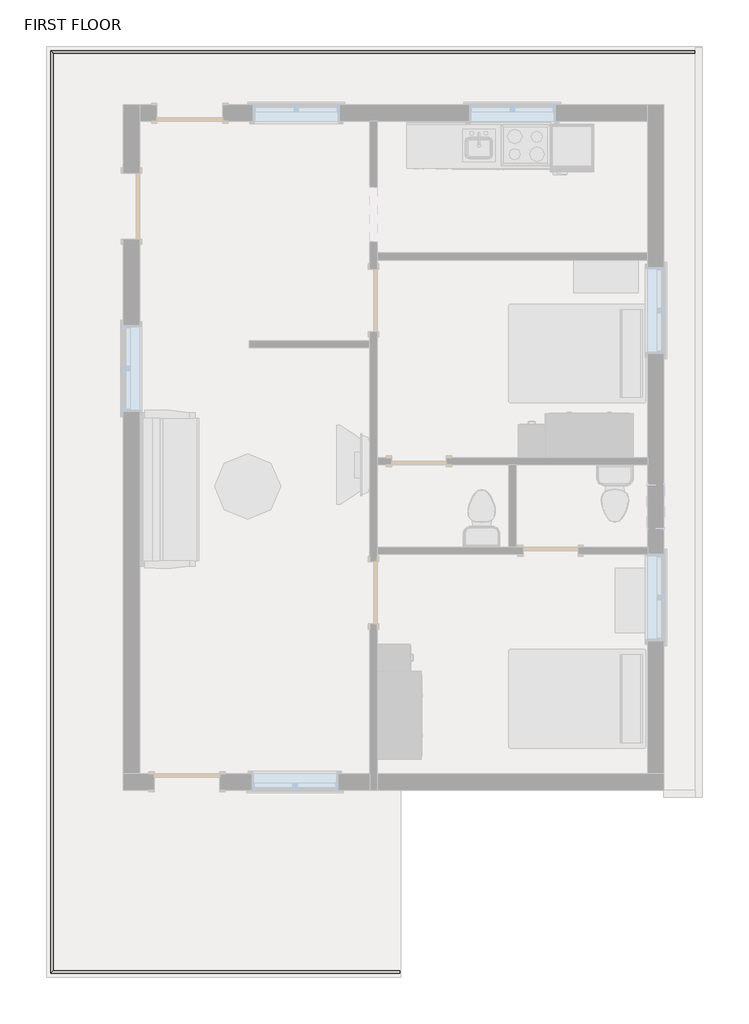
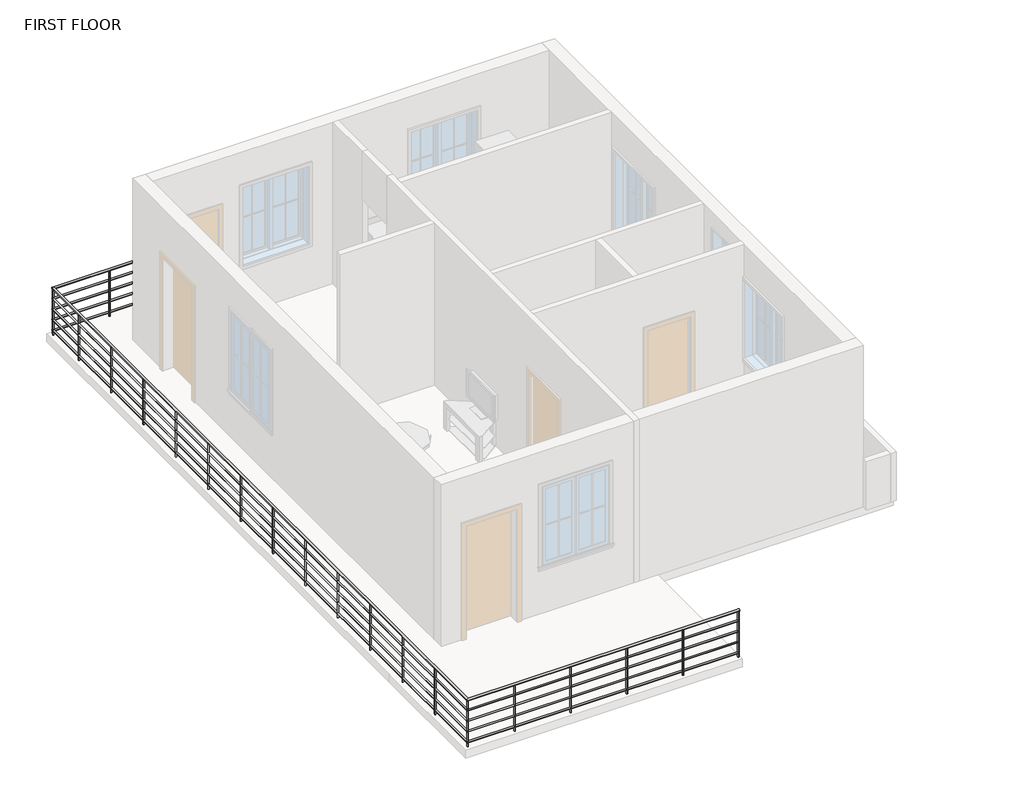
# One storey, part 2 of 3: 1 railing.
"""IFC4 building model written with IfcOpenShell, lengths in millimetres."""

from ifc_helpers import new_model, si_unit, point, frame, frame_2d, origin, place, context, project, spatial, circle_curve, ellipse_curve, trimmed, segment, composite_curve, outline, extrude, element, save
from ifc_brep_helpers import plane_surface, cylinder_surface, advanced_brep

model = new_model("IFC4")

# Units and contexts
model_context = context("Model", 3, world=origin())
ifc_project = project(units=[si_unit("LENGTHUNIT", "METRE", prefix="MILLI")], contexts=[model_context])

# Site, building, storey
site = spatial("IfcSite", under=ifc_project)
building = spatial("IfcBuilding", under=site)
storey = spatial("IfcBuildingStorey", under=building, Name="FIRST FLOOR", Elevation=3200.4)

# Railing
placement = place(None, origin())
element("IfcRailing", 1, ObjectType="900mm Pipe", at=placement, inside=storey, context=model_context, shape_type="SolidModel", body=[
    advanced_brep(
    [(200.9145071, -6925.6741001, 4080.4), (200.9145071, -6965.6741001, 4080.4), (-4655.4544048, -6965.6741001, 4080.4), (-4615.4544048, -6925.6741001, 4080.4), (-4655.4544048, 5865.7351347, 4080.4), (-4615.4544048, 5825.7351347, 4080.4), (4406.9455952, 5825.7351347, 4080.4), (4406.9455952, 5865.7351347, 4080.4)],
    [
        (0, 1, circle_curve(frame((200.9145071, -6945.6741001, 4080.4), z_axis=(1.0, 0.0, 0.0), x_axis=(0.0, -1.0, 0.0)), 20.0)),
        (1, 0, circle_curve(frame((200.9145071, -6945.6741001, 4080.4), z_axis=(1.0, 0.0, 0.0), x_axis=(0.0, -1.0, 0.0)), 20.0)),
        (1, 2),
        (2, 3, ellipse_curve(frame((-4635.4544048, -6945.6741001, 4080.4), z_axis=(0.7071067811865458, -0.7071067811865492, 0.0), x_axis=(0.7071067811865492, 0.7071067811865458, 0.0)), 28.2842712, 20.0)),
        (3, 0),
        (3, 2, ellipse_curve(frame((-4635.4544048, -6945.6741001, 4080.4), z_axis=(0.7071067811865458, -0.7071067811865492, 0.0), x_axis=(0.7071067811865492, 0.7071067811865458, 0.0)), 28.2842712, 20.0)),
        (2, 4),
        (4, 5, ellipse_curve(frame((-4635.4544048, 5845.7351347, 4080.4), z_axis=(-0.7071067811865491, -0.7071067811865459, 0.0), x_axis=(0.7071067811865458, -0.7071067811865491, 0.0)), 28.2842712, 20.0)),
        (5, 3),
        (5, 4, ellipse_curve(frame((-4635.4544048, 5845.7351347, 4080.4), z_axis=(-0.7071067811865491, -0.7071067811865459, 0.0), x_axis=(0.7071067811865458, -0.7071067811865491, 0.0)), 28.2842712, 20.0)),
        (6, 7, circle_curve(frame((4406.9455952, 5845.7351347, 4080.4), z_axis=(1.0, 0.0, 0.0), x_axis=(0.0, 1.0, 0.0)), 20.0)),
        (7, 6, circle_curve(frame((4406.9455952, 5845.7351347, 4080.4), z_axis=(1.0, 0.0, 0.0), x_axis=(0.0, 1.0, 0.0)), 20.0)),
        (4, 7),
        (6, 5),
    ],
    [
        plane_surface(frame((200.9145071, -6945.6741001, 4100.4), z_axis=(1.0, 0.0, 0.0), x_axis=(0.0, -1.0, 0.0))),
        cylinder_surface(frame((200.9145071, -6945.6741001, 4080.4), z_axis=(1.0, 0.0, 0.0), x_axis=(0.0, -1.0, 0.0)), 20.0),
        cylinder_surface(frame((-4635.4544048, -6945.6741001, 4080.4), z_axis=(0.0, -1.0, 0.0), x_axis=(-1.0, 0.0, 0.0)), 20.0),
        plane_surface(frame((4406.9455952, 5845.7351347, 4100.4), z_axis=(1.0, 0.0, 0.0), x_axis=(0.0, 1.0, 0.0))),
        cylinder_surface(frame((-4635.4544048, 5845.7351347, 4080.4), z_axis=(-1.0, 0.0, 0.0), x_axis=(0.0, 1.0, 0.0)), 20.0),
    ],
    [
        (0, [[1, 2]]),
        (1, [[-2, 3, 4, 5]]),
        (1, [[-1, -5, 6, -3]]),
        (2, [[-4, 7, 8, 9]]),
        (2, [[-6, -9, 10, -7]]),
        (3, [[11, 12]]),
        (4, [[-8, 13, -11, 14]]),
        (4, [[-10, -14, -12, -13]]),
    ],
),
    advanced_brep(
    [(200.9145071, -6960.6741001, 3885.4), (200.9145071, -6930.6741001, 3885.4), (4406.9455952, 5860.7351347, 3885.4), (4406.9455952, 5830.7351347, 3885.4), (-4650.4544048, -6960.6741001, 3885.4), (-4620.4544048, -6930.6741001, 3885.4), (-4650.4544048, 5860.7351347, 3885.4), (-4620.4544048, 5830.7351347, 3885.4)],
    [
        (0, 1, circle_curve(frame((200.9145071, -6945.6741001, 3885.4), z_axis=(1.0, 0.0, 0.0), x_axis=(0.0, 1.0, 0.0)), 15.0)),
        (1, 0, circle_curve(frame((200.9145071, -6945.6741001, 3885.4), z_axis=(1.0, 0.0, 0.0), x_axis=(0.0, 1.0, 0.0)), 15.0)),
        (2, 3, circle_curve(frame((4406.9455952, 5845.7351347, 3885.4), z_axis=(1.0, 0.0, 0.0), x_axis=(0.0, -1.0, 0.0)), 15.0)),
        (3, 2, circle_curve(frame((4406.9455952, 5845.7351347, 3885.4), z_axis=(1.0, 0.0, 0.0), x_axis=(0.0, -1.0, 0.0)), 15.0)),
        (0, 4),
        (4, 5, ellipse_curve(frame((-4635.4544048, -6945.6741001, 3885.4), z_axis=(0.7071067811865458, -0.7071067811865492, 0.0), x_axis=(0.7071067811865492, 0.7071067811865458, 0.0)), 21.2132034, 15.0)),
        (5, 1),
        (5, 4, ellipse_curve(frame((-4635.4544048, -6945.6741001, 3885.4), z_axis=(0.7071067811865458, -0.7071067811865492, 0.0), x_axis=(0.7071067811865492, 0.7071067811865458, 0.0)), 21.2132034, 15.0)),
        (4, 6),
        (6, 7, ellipse_curve(frame((-4635.4544048, 5845.7351347, 3885.4), z_axis=(-0.7071067811865491, -0.7071067811865459, 0.0), x_axis=(0.7071067811865458, -0.7071067811865491, 0.0)), 21.2132034, 15.0)),
        (7, 5),
        (7, 6, ellipse_curve(frame((-4635.4544048, 5845.7351347, 3885.4), z_axis=(-0.7071067811865491, -0.7071067811865459, 0.0), x_axis=(0.7071067811865458, -0.7071067811865491, 0.0)), 21.2132034, 15.0)),
        (6, 2),
        (3, 7),
    ],
    [
        plane_surface(frame((200.9145071, -6945.6741001, 3900.4), z_axis=(1.0, 0.0, 0.0), x_axis=(0.0, -1.0, 0.0))),
        plane_surface(frame((4406.9455952, 5845.7351347, 3900.4), z_axis=(1.0, 0.0, 0.0), x_axis=(0.0, 1.0, 0.0))),
        cylinder_surface(frame((200.9145071, -6945.6741001, 3885.4), z_axis=(1.0, 0.0, 0.0), x_axis=(0.0, 1.0, 0.0)), 15.0),
        cylinder_surface(frame((-4635.4544048, -6945.6741001, 3885.4), z_axis=(0.0, -1.0, 0.0), x_axis=(1.0, 0.0, 0.0)), 15.0),
        cylinder_surface(frame((-4635.4544048, 5845.7351347, 3885.4), z_axis=(-1.0, 0.0, 0.0), x_axis=(0.0, -1.0, 0.0)), 15.0),
    ],
    [
        (0, [[1, 2]]),
        (1, [[3, 4]]),
        (2, [[-1, 5, 6, 7]]),
        (2, [[-2, -7, 8, -5]]),
        (3, [[-6, 9, 10, 11]]),
        (3, [[-8, -11, 12, -9]]),
        (4, [[-10, 13, -4, 14]]),
        (4, [[-12, -14, -3, -13]]),
    ],
),
    advanced_brep(
    [(200.9145071, -6960.6741001, 3685.4), (200.9145071, -6930.6741001, 3685.4), (4406.9455952, 5860.7351347, 3685.4), (4406.9455952, 5830.7351347, 3685.4), (-4650.4544048, -6960.6741001, 3685.4), (-4620.4544048, -6930.6741001, 3685.4), (-4650.4544048, 5860.7351347, 3685.4), (-4620.4544048, 5830.7351347, 3685.4)],
    [
        (0, 1, circle_curve(frame((200.9145071, -6945.6741001, 3685.4), z_axis=(1.0, 0.0, 0.0), x_axis=(0.0, 1.0, 0.0)), 15.0)),
        (1, 0, circle_curve(frame((200.9145071, -6945.6741001, 3685.4), z_axis=(1.0, 0.0, 0.0), x_axis=(0.0, 1.0, 0.0)), 15.0)),
        (2, 3, circle_curve(frame((4406.9455952, 5845.7351347, 3685.4), z_axis=(1.0, 0.0, 0.0), x_axis=(0.0, -1.0, 0.0)), 15.0)),
        (3, 2, circle_curve(frame((4406.9455952, 5845.7351347, 3685.4), z_axis=(1.0, 0.0, 0.0), x_axis=(0.0, -1.0, 0.0)), 15.0)),
        (0, 4),
        (4, 5, ellipse_curve(frame((-4635.4544048, -6945.6741001, 3685.4), z_axis=(0.7071067811865458, -0.7071067811865492, 0.0), x_axis=(0.7071067811865492, 0.7071067811865458, 0.0)), 21.2132034, 15.0)),
        (5, 1),
        (5, 4, ellipse_curve(frame((-4635.4544048, -6945.6741001, 3685.4), z_axis=(0.7071067811865458, -0.7071067811865492, 0.0), x_axis=(0.7071067811865492, 0.7071067811865458, 0.0)), 21.2132034, 15.0)),
        (4, 6),
        (6, 7, ellipse_curve(frame((-4635.4544048, 5845.7351347, 3685.4), z_axis=(-0.7071067811865491, -0.7071067811865459, 0.0), x_axis=(0.7071067811865458, -0.7071067811865491, 0.0)), 21.2132034, 15.0)),
        (7, 5),
        (7, 6, ellipse_curve(frame((-4635.4544048, 5845.7351347, 3685.4), z_axis=(-0.7071067811865491, -0.7071067811865459, 0.0), x_axis=(0.7071067811865458, -0.7071067811865491, 0.0)), 21.2132034, 15.0)),
        (6, 2),
        (3, 7),
    ],
    [
        plane_surface(frame((200.9145071, -6945.6741001, 3700.4), z_axis=(1.0, 0.0, 0.0), x_axis=(0.0, -1.0, 0.0))),
        plane_surface(frame((4406.9455952, 5845.7351347, 3700.4), z_axis=(1.0, 0.0, 0.0), x_axis=(0.0, 1.0, 0.0))),
        cylinder_surface(frame((200.9145071, -6945.6741001, 3685.4), z_axis=(1.0, 0.0, 0.0), x_axis=(0.0, 1.0, 0.0)), 15.0),
        cylinder_surface(frame((-4635.4544048, -6945.6741001, 3685.4), z_axis=(0.0, -1.0, 0.0), x_axis=(1.0, 0.0, 0.0)), 15.0),
        cylinder_surface(frame((-4635.4544048, 5845.7351347, 3685.4), z_axis=(-1.0, 0.0, 0.0), x_axis=(0.0, -1.0, 0.0)), 15.0),
    ],
    [
        (0, [[1, 2]]),
        (1, [[3, 4]]),
        (2, [[-1, 5, 6, 7]]),
        (2, [[-2, -7, 8, -5]]),
        (3, [[-6, 9, 10, 11]]),
        (3, [[-8, -11, 12, -9]]),
        (4, [[-10, 13, -4, 14]]),
        (4, [[-12, -14, -3, -13]]),
    ],
),
    advanced_brep(
    [(200.9145071, -6960.6741001, 3485.4), (200.9145071, -6930.6741001, 3485.4), (-4650.4544048, -6960.6741001, 3485.4), (-4620.4544048, -6930.6741001, 3485.4), (-4650.4544048, 5860.7351347, 3485.4), (-4620.4544048, 5830.7351347, 3485.4), (4406.9455952, 5860.7351347, 3485.4), (4406.9455952, 5830.7351347, 3485.4)],
    [
        (0, 1, circle_curve(frame((200.9145071, -6945.6741001, 3485.4), z_axis=(1.0, 0.0, 0.0), x_axis=(0.0, 1.0, 0.0)), 15.0)),
        (1, 0, circle_curve(frame((200.9145071, -6945.6741001, 3485.4), z_axis=(1.0, 0.0, 0.0), x_axis=(0.0, 1.0, 0.0)), 15.0)),
        (0, 2),
        (2, 3, ellipse_curve(frame((-4635.4544048, -6945.6741001, 3485.4), z_axis=(0.7071067811865458, -0.7071067811865492, 0.0), x_axis=(0.7071067811865492, 0.7071067811865458, 0.0)), 21.2132034, 15.0)),
        (3, 1),
        (3, 2, ellipse_curve(frame((-4635.4544048, -6945.6741001, 3485.4), z_axis=(0.7071067811865458, -0.7071067811865492, 0.0), x_axis=(0.7071067811865492, 0.7071067811865458, 0.0)), 21.2132034, 15.0)),
        (2, 4),
        (4, 5, ellipse_curve(frame((-4635.4544048, 5845.7351347, 3485.4), z_axis=(-0.7071067811865491, -0.7071067811865459, 0.0), x_axis=(0.7071067811865458, -0.7071067811865491, 0.0)), 21.2132034, 15.0)),
        (5, 3),
        (5, 4, ellipse_curve(frame((-4635.4544048, 5845.7351347, 3485.4), z_axis=(-0.7071067811865491, -0.7071067811865459, 0.0), x_axis=(0.7071067811865458, -0.7071067811865491, 0.0)), 21.2132034, 15.0)),
        (6, 7, circle_curve(frame((4406.9455952, 5845.7351347, 3485.4), z_axis=(1.0, 0.0, 0.0), x_axis=(0.0, -1.0, 0.0)), 15.0)),
        (7, 6, circle_curve(frame((4406.9455952, 5845.7351347, 3485.4), z_axis=(1.0, 0.0, 0.0), x_axis=(0.0, -1.0, 0.0)), 15.0)),
        (4, 6),
        (7, 5),
    ],
    [
        plane_surface(frame((200.9145071, -6945.6741001, 3500.4), z_axis=(1.0, 0.0, 0.0), x_axis=(0.0, -1.0, 0.0))),
        cylinder_surface(frame((200.9145071, -6945.6741001, 3485.4), z_axis=(1.0, 0.0, 0.0), x_axis=(0.0, 1.0, 0.0)), 15.0),
        cylinder_surface(frame((-4635.4544048, -6945.6741001, 3485.4), z_axis=(0.0, -1.0, 0.0), x_axis=(1.0, 0.0, 0.0)), 15.0),
        plane_surface(frame((4406.9455952, 5845.7351347, 3500.4), z_axis=(1.0, 0.0, 0.0), x_axis=(0.0, 1.0, 0.0))),
        cylinder_surface(frame((-4635.4544048, 5845.7351347, 3485.4), z_axis=(-1.0, 0.0, 0.0), x_axis=(0.0, -1.0, 0.0)), 15.0),
    ],
    [
        (0, [[1, 2]]),
        (1, [[-1, 3, 4, 5]]),
        (1, [[-2, -5, 6, -3]]),
        (2, [[-4, 7, 8, 9]]),
        (2, [[-6, -9, 10, -7]]),
        (3, [[11, 12]]),
        (4, [[-8, 13, -12, 14]]),
        (4, [[-10, -14, -11, -13]]),
    ],
),
    advanced_brep(
    [(200.9145071, -6960.6741001, 3285.4), (200.9145071, -6930.6741001, 3285.4), (-4650.4544048, -6960.6741001, 3285.4), (-4620.4544048, -6930.6741001, 3285.4), (-4650.4544048, 5860.7351347, 3285.4), (-4620.4544048, 5830.7351347, 3285.4), (4406.9455952, 5860.7351347, 3285.4), (4406.9455952, 5830.7351347, 3285.4)],
    [
        (0, 1, circle_curve(frame((200.9145071, -6945.6741001, 3285.4), z_axis=(1.0, 0.0, 0.0), x_axis=(0.0, 1.0, 0.0)), 15.0)),
        (1, 0, circle_curve(frame((200.9145071, -6945.6741001, 3285.4), z_axis=(1.0, 0.0, 0.0), x_axis=(0.0, 1.0, 0.0)), 15.0)),
        (0, 2),
        (2, 3, ellipse_curve(frame((-4635.4544048, -6945.6741001, 3285.4), z_axis=(0.7071067811865458, -0.7071067811865492, 0.0), x_axis=(0.7071067811865492, 0.7071067811865458, 0.0)), 21.2132034, 15.0)),
        (3, 1),
        (3, 2, ellipse_curve(frame((-4635.4544048, -6945.6741001, 3285.4), z_axis=(0.7071067811865458, -0.7071067811865492, 0.0), x_axis=(0.7071067811865492, 0.7071067811865458, 0.0)), 21.2132034, 15.0)),
        (2, 4),
        (4, 5, ellipse_curve(frame((-4635.4544048, 5845.7351347, 3285.4), z_axis=(-0.7071067811865491, -0.7071067811865459, 0.0), x_axis=(0.7071067811865458, -0.7071067811865491, 0.0)), 21.2132034, 15.0)),
        (5, 3),
        (5, 4, ellipse_curve(frame((-4635.4544048, 5845.7351347, 3285.4), z_axis=(-0.7071067811865491, -0.7071067811865459, 0.0), x_axis=(0.7071067811865458, -0.7071067811865491, 0.0)), 21.2132034, 15.0)),
        (6, 7, circle_curve(frame((4406.9455952, 5845.7351347, 3285.4), z_axis=(1.0, 0.0, 0.0), x_axis=(0.0, -1.0, 0.0)), 15.0)),
        (7, 6, circle_curve(frame((4406.9455952, 5845.7351347, 3285.4), z_axis=(1.0, 0.0, 0.0), x_axis=(0.0, -1.0, 0.0)), 15.0)),
        (4, 6),
        (7, 5),
    ],
    [
        plane_surface(frame((200.9145071, -6945.6741001, 3300.4), z_axis=(1.0, 0.0, 0.0), x_axis=(0.0, -1.0, 0.0))),
        cylinder_surface(frame((200.9145071, -6945.6741001, 3285.4), z_axis=(1.0, 0.0, 0.0), x_axis=(0.0, 1.0, 0.0)), 15.0),
        cylinder_surface(frame((-4635.4544048, -6945.6741001, 3285.4), z_axis=(0.0, -1.0, 0.0), x_axis=(1.0, 0.0, 0.0)), 15.0),
        plane_surface(frame((4406.9455952, 5845.7351347, 3300.4), z_axis=(1.0, 0.0, 0.0), x_axis=(0.0, 1.0, 0.0))),
        cylinder_surface(frame((-4635.4544048, 5845.7351347, 3285.4), z_axis=(-1.0, 0.0, 0.0), x_axis=(0.0, -1.0, 0.0)), 15.0),
    ],
    [
        (0, [[1, 2]]),
        (1, [[-1, 3, 4, 5]]),
        (1, [[-2, -5, 6, -3]]),
        (2, [[-4, 7, 8, 9]]),
        (2, [[-6, -9, 10, -7]]),
        (3, [[11, 12]]),
        (4, [[-8, 13, -12, 14]]),
        (4, [[-10, -14, -11, -13]]),
    ],
),
    extrude(outline(composite_curve([segment(trimmed(circle_curve(frame_2d((4364.5455952, 5845.7351347)), 12.5), [point((4364.5455952, 5858.2351347))], [point((4364.5455952, 5833.2351347))], False, "CARTESIAN"), True, "CONTINUOUS"), segment(trimmed(circle_curve(frame_2d((4364.5455952, 5845.7351347)), 12.5), [point((4364.5455952, 5833.2351347))], [point((4364.5455952, 5858.2351347))], False, "CARTESIAN"), True, "CONTINUOUS")], self_intersect=False)), frame((0.0, 0.0, 3200.4), z_axis=(0.0, 0.0, 1.0), x_axis=(1.0, 0.0, 0.0)), (0.0, 0.0, 1.0), 860.0),
    extrude(outline(composite_curve([segment(trimmed(circle_curve(frame_2d((3364.5455952, 5845.7351347)), 12.5), [point((3364.5455952, 5858.2351347))], [point((3364.5455952, 5833.2351347))], False, "CARTESIAN"), True, "CONTINUOUS"), segment(trimmed(circle_curve(frame_2d((3364.5455952, 5845.7351347)), 12.5), [point((3364.5455952, 5833.2351347))], [point((3364.5455952, 5858.2351347))], False, "CARTESIAN"), True, "CONTINUOUS")], self_intersect=False)), frame((0.0, 0.0, 3200.4), z_axis=(0.0, 0.0, 1.0), x_axis=(1.0, 0.0, 0.0)), (0.0, 0.0, 1.0), 860.0),
    extrude(outline(composite_curve([segment(trimmed(circle_curve(frame_2d((2364.5455952, 5845.7351347)), 12.5), [point((2364.5455952, 5858.2351347))], [point((2364.5455952, 5833.2351347))], False, "CARTESIAN"), True, "CONTINUOUS"), segment(trimmed(circle_curve(frame_2d((2364.5455952, 5845.7351347)), 12.5), [point((2364.5455952, 5833.2351347))], [point((2364.5455952, 5858.2351347))], False, "CARTESIAN"), True, "CONTINUOUS")], self_intersect=False)), frame((0.0, 0.0, 3200.4), z_axis=(0.0, 0.0, 1.0), x_axis=(1.0, 0.0, 0.0)), (0.0, 0.0, 1.0), 860.0),
    extrude(outline(composite_curve([segment(trimmed(circle_curve(frame_2d((1364.5455952, 5845.7351347)), 12.5), [point((1364.5455952, 5858.2351347))], [point((1364.5455952, 5833.2351347))], False, "CARTESIAN"), True, "CONTINUOUS"), segment(trimmed(circle_curve(frame_2d((1364.5455952, 5845.7351347)), 12.5), [point((1364.5455952, 5833.2351347))], [point((1364.5455952, 5858.2351347))], False, "CARTESIAN"), True, "CONTINUOUS")], self_intersect=False)), frame((0.0, 0.0, 3200.4), z_axis=(0.0, 0.0, 1.0), x_axis=(1.0, 0.0, 0.0)), (0.0, 0.0, 1.0), 860.0),
    extrude(outline(composite_curve([segment(trimmed(circle_curve(frame_2d((364.5455952, 5845.7351347)), 12.5), [point((364.5455952, 5858.2351347))], [point((364.5455952, 5833.2351347))], False, "CARTESIAN"), True, "CONTINUOUS"), segment(trimmed(circle_curve(frame_2d((364.5455952, 5845.7351347)), 12.5), [point((364.5455952, 5833.2351347))], [point((364.5455952, 5858.2351347))], False, "CARTESIAN"), True, "CONTINUOUS")], self_intersect=False)), frame((0.0, 0.0, 3200.4), z_axis=(0.0, 0.0, 1.0), x_axis=(1.0, 0.0, 0.0)), (0.0, 0.0, 1.0), 860.0),
    extrude(outline(composite_curve([segment(trimmed(circle_curve(frame_2d((-635.4544048, 5845.7351347)), 12.5), [point((-635.4544048, 5858.2351347))], [point((-635.4544048, 5833.2351347))], False, "CARTESIAN"), True, "CONTINUOUS"), segment(trimmed(circle_curve(frame_2d((-635.4544048, 5845.7351347)), 12.5), [point((-635.4544048, 5833.2351347))], [point((-635.4544048, 5858.2351347))], False, "CARTESIAN"), True, "CONTINUOUS")], self_intersect=False)), frame((0.0, 0.0, 3200.4), z_axis=(0.0, 0.0, 1.0), x_axis=(1.0, 0.0, 0.0)), (0.0, 0.0, 1.0), 860.0),
    extrude(outline(composite_curve([segment(trimmed(circle_curve(frame_2d((-1635.4544048, 5845.7351347)), 12.5), [point((-1635.4544048, 5858.2351347))], [point((-1635.4544048, 5833.2351347))], False, "CARTESIAN"), True, "CONTINUOUS"), segment(trimmed(circle_curve(frame_2d((-1635.4544048, 5845.7351347)), 12.5), [point((-1635.4544048, 5833.2351347))], [point((-1635.4544048, 5858.2351347))], False, "CARTESIAN"), True, "CONTINUOUS")], self_intersect=False)), frame((0.0, 0.0, 3200.4), z_axis=(0.0, 0.0, 1.0), x_axis=(1.0, 0.0, 0.0)), (0.0, 0.0, 1.0), 860.0),
    extrude(outline(composite_curve([segment(trimmed(circle_curve(frame_2d((-2635.4544048, 5845.7351347)), 12.5), [point((-2635.4544048, 5858.2351347))], [point((-2635.4544048, 5833.2351347))], False, "CARTESIAN"), True, "CONTINUOUS"), segment(trimmed(circle_curve(frame_2d((-2635.4544048, 5845.7351347)), 12.5), [point((-2635.4544048, 5833.2351347))], [point((-2635.4544048, 5858.2351347))], False, "CARTESIAN"), True, "CONTINUOUS")], self_intersect=False)), frame((0.0, 0.0, 3200.4), z_axis=(0.0, 0.0, 1.0), x_axis=(1.0, 0.0, 0.0)), (0.0, 0.0, 1.0), 860.0),
    extrude(outline(composite_curve([segment(trimmed(circle_curve(frame_2d((-3635.4544048, 5845.7351347)), 12.5), [point((-3635.4544048, 5858.2351347))], [point((-3635.4544048, 5833.2351347))], False, "CARTESIAN"), True, "CONTINUOUS"), segment(trimmed(circle_curve(frame_2d((-3635.4544048, 5845.7351347)), 12.5), [point((-3635.4544048, 5833.2351347))], [point((-3635.4544048, 5858.2351347))], False, "CARTESIAN"), True, "CONTINUOUS")], self_intersect=False)), frame((0.0, 0.0, 3200.4), z_axis=(0.0, 0.0, 1.0), x_axis=(1.0, 0.0, 0.0)), (0.0, 0.0, 1.0), 860.0),
    extrude(outline(composite_curve([segment(trimmed(circle_curve(frame_2d((-4635.4544048, 5054.3258999)), 12.5), [point((-4647.9544048, 5054.3258999))], [point((-4622.9544048, 5054.3258999))], False, "CARTESIAN"), True, "CONTINUOUS"), segment(trimmed(circle_curve(frame_2d((-4635.4544048, 5054.3258999)), 12.5), [point((-4622.9544048, 5054.3258999))], [point((-4647.9544048, 5054.3258999))], False, "CARTESIAN"), True, "CONTINUOUS")], self_intersect=False)), frame((0.0, 0.0, 3200.4), z_axis=(0.0, 0.0, 1.0), x_axis=(1.0, 0.0, 0.0)), (0.0, 0.0, 1.0), 860.0),
    extrude(outline(composite_curve([segment(trimmed(circle_curve(frame_2d((-4635.4544048, 4054.3258999)), 12.5), [point((-4647.9544048, 4054.3258999))], [point((-4622.9544048, 4054.3258999))], False, "CARTESIAN"), True, "CONTINUOUS"), segment(trimmed(circle_curve(frame_2d((-4635.4544048, 4054.3258999)), 12.5), [point((-4622.9544048, 4054.3258999))], [point((-4647.9544048, 4054.3258999))], False, "CARTESIAN"), True, "CONTINUOUS")], self_intersect=False)), frame((0.0, 0.0, 3200.4), z_axis=(0.0, 0.0, 1.0), x_axis=(1.0, 0.0, 0.0)), (0.0, 0.0, 1.0), 860.0),
    extrude(outline(composite_curve([segment(trimmed(circle_curve(frame_2d((-4635.4544048, 3054.3258999)), 12.5), [point((-4647.9544048, 3054.3258999))], [point((-4622.9544048, 3054.3258999))], False, "CARTESIAN"), True, "CONTINUOUS"), segment(trimmed(circle_curve(frame_2d((-4635.4544048, 3054.3258999)), 12.5), [point((-4622.9544048, 3054.3258999))], [point((-4647.9544048, 3054.3258999))], False, "CARTESIAN"), True, "CONTINUOUS")], self_intersect=False)), frame((0.0, 0.0, 3200.4), z_axis=(0.0, 0.0, 1.0), x_axis=(1.0, 0.0, 0.0)), (0.0, 0.0, 1.0), 860.0),
    extrude(outline(composite_curve([segment(trimmed(circle_curve(frame_2d((-4635.4544048, 2054.3258999)), 12.5), [point((-4647.9544048, 2054.3258999))], [point((-4622.9544048, 2054.3258999))], False, "CARTESIAN"), True, "CONTINUOUS"), segment(trimmed(circle_curve(frame_2d((-4635.4544048, 2054.3258999)), 12.5), [point((-4622.9544048, 2054.3258999))], [point((-4647.9544048, 2054.3258999))], False, "CARTESIAN"), True, "CONTINUOUS")], self_intersect=False)), frame((0.0, 0.0, 3200.4), z_axis=(0.0, 0.0, 1.0), x_axis=(1.0, 0.0, 0.0)), (0.0, 0.0, 1.0), 860.0),
    extrude(outline(composite_curve([segment(trimmed(circle_curve(frame_2d((-4635.4544048, 1054.3258999)), 12.5), [point((-4647.9544048, 1054.3258999))], [point((-4622.9544048, 1054.3258999))], False, "CARTESIAN"), True, "CONTINUOUS"), segment(trimmed(circle_curve(frame_2d((-4635.4544048, 1054.3258999)), 12.5), [point((-4622.9544048, 1054.3258999))], [point((-4647.9544048, 1054.3258999))], False, "CARTESIAN"), True, "CONTINUOUS")], self_intersect=False)), frame((0.0, 0.0, 3200.4), z_axis=(0.0, 0.0, 1.0), x_axis=(1.0, 0.0, 0.0)), (0.0, 0.0, 1.0), 860.0),
    extrude(outline(composite_curve([segment(trimmed(circle_curve(frame_2d((-4635.4544048, 54.3258999)), 12.5), [point((-4647.9544048, 54.3258999))], [point((-4622.9544048, 54.3258999))], False, "CARTESIAN"), True, "CONTINUOUS"), segment(trimmed(circle_curve(frame_2d((-4635.4544048, 54.3258999)), 12.5), [point((-4622.9544048, 54.3258999))], [point((-4647.9544048, 54.3258999))], False, "CARTESIAN"), True, "CONTINUOUS")], self_intersect=False)), frame((0.0, 0.0, 3200.4), z_axis=(0.0, 0.0, 1.0), x_axis=(1.0, 0.0, 0.0)), (0.0, 0.0, 1.0), 860.0),
    extrude(outline(composite_curve([segment(trimmed(circle_curve(frame_2d((-4635.4544048, -945.6741001)), 12.5), [point((-4647.9544048, -945.6741001))], [point((-4622.9544048, -945.6741001))], False, "CARTESIAN"), True, "CONTINUOUS"), segment(trimmed(circle_curve(frame_2d((-4635.4544048, -945.6741001)), 12.5), [point((-4622.9544048, -945.6741001))], [point((-4647.9544048, -945.6741001))], False, "CARTESIAN"), True, "CONTINUOUS")], self_intersect=False)), frame((0.0, 0.0, 3200.4), z_axis=(0.0, 0.0, 1.0), x_axis=(1.0, 0.0, 0.0)), (0.0, 0.0, 1.0), 860.0),
    extrude(outline(composite_curve([segment(trimmed(circle_curve(frame_2d((-4635.4544048, -1945.6741001)), 12.5), [point((-4647.9544048, -1945.6741001))], [point((-4622.9544048, -1945.6741001))], False, "CARTESIAN"), True, "CONTINUOUS"), segment(trimmed(circle_curve(frame_2d((-4635.4544048, -1945.6741001)), 12.5), [point((-4622.9544048, -1945.6741001))], [point((-4647.9544048, -1945.6741001))], False, "CARTESIAN"), True, "CONTINUOUS")], self_intersect=False)), frame((0.0, 0.0, 3200.4), z_axis=(0.0, 0.0, 1.0), x_axis=(1.0, 0.0, 0.0)), (0.0, 0.0, 1.0), 860.0),
    extrude(outline(composite_curve([segment(trimmed(circle_curve(frame_2d((-4635.4544048, -2945.6741001)), 12.5), [point((-4647.9544048, -2945.6741001))], [point((-4622.9544048, -2945.6741001))], False, "CARTESIAN"), True, "CONTINUOUS"), segment(trimmed(circle_curve(frame_2d((-4635.4544048, -2945.6741001)), 12.5), [point((-4622.9544048, -2945.6741001))], [point((-4647.9544048, -2945.6741001))], False, "CARTESIAN"), True, "CONTINUOUS")], self_intersect=False)), frame((0.0, 0.0, 3200.4), z_axis=(0.0, 0.0, 1.0), x_axis=(1.0, 0.0, 0.0)), (0.0, 0.0, 1.0), 860.0),
    extrude(outline(composite_curve([segment(trimmed(circle_curve(frame_2d((-4635.4544048, -3945.6741001)), 12.5), [point((-4647.9544048, -3945.6741001))], [point((-4622.9544048, -3945.6741001))], False, "CARTESIAN"), True, "CONTINUOUS"), segment(trimmed(circle_curve(frame_2d((-4635.4544048, -3945.6741001)), 12.5), [point((-4622.9544048, -3945.6741001))], [point((-4647.9544048, -3945.6741001))], False, "CARTESIAN"), True, "CONTINUOUS")], self_intersect=False)), frame((0.0, 0.0, 3200.4), z_axis=(0.0, 0.0, 1.0), x_axis=(1.0, 0.0, 0.0)), (0.0, 0.0, 1.0), 860.0),
    extrude(outline(composite_curve([segment(trimmed(circle_curve(frame_2d((-4635.4544048, -4945.6741001)), 12.5), [point((-4647.9544048, -4945.6741001))], [point((-4622.9544048, -4945.6741001))], False, "CARTESIAN"), True, "CONTINUOUS"), segment(trimmed(circle_curve(frame_2d((-4635.4544048, -4945.6741001)), 12.5), [point((-4622.9544048, -4945.6741001))], [point((-4647.9544048, -4945.6741001))], False, "CARTESIAN"), True, "CONTINUOUS")], self_intersect=False)), frame((0.0, 0.0, 3200.4), z_axis=(0.0, 0.0, 1.0), x_axis=(1.0, 0.0, 0.0)), (0.0, 0.0, 1.0), 860.0),
    extrude(outline(composite_curve([segment(trimmed(circle_curve(frame_2d((-4635.4544048, -5945.6741001)), 12.5), [point((-4647.9544048, -5945.6741001))], [point((-4622.9544048, -5945.6741001))], False, "CARTESIAN"), True, "CONTINUOUS"), segment(trimmed(circle_curve(frame_2d((-4635.4544048, -5945.6741001)), 12.5), [point((-4622.9544048, -5945.6741001))], [point((-4647.9544048, -5945.6741001))], False, "CARTESIAN"), True, "CONTINUOUS")], self_intersect=False)), frame((0.0, 0.0, 3200.4), z_axis=(0.0, 0.0, 1.0), x_axis=(1.0, 0.0, 0.0)), (0.0, 0.0, 1.0), 860.0),
    extrude(outline(composite_curve([segment(trimmed(circle_curve(frame_2d((-3799.0854929, -6945.6741001)), 12.5), [point((-3799.0854929, -6958.1741001))], [point((-3799.0854929, -6933.1741001))], False, "CARTESIAN"), True, "CONTINUOUS"), segment(trimmed(circle_curve(frame_2d((-3799.0854929, -6945.6741001)), 12.5), [point((-3799.0854929, -6933.1741001))], [point((-3799.0854929, -6958.1741001))], False, "CARTESIAN"), True, "CONTINUOUS")], self_intersect=False)), frame((0.0, 0.0, 3200.4), z_axis=(0.0, 0.0, 1.0), x_axis=(1.0, 0.0, 0.0)), (0.0, 0.0, 1.0), 860.0),
    extrude(outline(composite_curve([segment(trimmed(circle_curve(frame_2d((-2799.0854929, -6945.6741001)), 12.5), [point((-2799.0854929, -6958.1741001))], [point((-2799.0854929, -6933.1741001))], False, "CARTESIAN"), True, "CONTINUOUS"), segment(trimmed(circle_curve(frame_2d((-2799.0854929, -6945.6741001)), 12.5), [point((-2799.0854929, -6933.1741001))], [point((-2799.0854929, -6958.1741001))], False, "CARTESIAN"), True, "CONTINUOUS")], self_intersect=False)), frame((0.0, 0.0, 3200.4), z_axis=(0.0, 0.0, 1.0), x_axis=(1.0, 0.0, 0.0)), (0.0, 0.0, 1.0), 860.0),
    extrude(outline(composite_curve([segment(trimmed(circle_curve(frame_2d((-1799.0854929, -6945.6741001)), 12.5), [point((-1799.0854929, -6958.1741001))], [point((-1799.0854929, -6933.1741001))], False, "CARTESIAN"), True, "CONTINUOUS"), segment(trimmed(circle_curve(frame_2d((-1799.0854929, -6945.6741001)), 12.5), [point((-1799.0854929, -6933.1741001))], [point((-1799.0854929, -6958.1741001))], False, "CARTESIAN"), True, "CONTINUOUS")], self_intersect=False)), frame((0.0, 0.0, 3200.4), z_axis=(0.0, 0.0, 1.0), x_axis=(1.0, 0.0, 0.0)), (0.0, 0.0, 1.0), 860.0),
    extrude(outline(composite_curve([segment(trimmed(circle_curve(frame_2d((-799.0854929, -6945.6741001)), 12.5), [point((-799.0854929, -6958.1741001))], [point((-799.0854929, -6933.1741001))], False, "CARTESIAN"), True, "CONTINUOUS"), segment(trimmed(circle_curve(frame_2d((-799.0854929, -6945.6741001)), 12.5), [point((-799.0854929, -6933.1741001))], [point((-799.0854929, -6958.1741001))], False, "CARTESIAN"), True, "CONTINUOUS")], self_intersect=False)), frame((0.0, 0.0, 3200.4), z_axis=(0.0, 0.0, 1.0), x_axis=(1.0, 0.0, 0.0)), (0.0, 0.0, 1.0), 860.0),
    extrude(outline(composite_curve([segment(trimmed(circle_curve(frame_2d((-4635.4544048, 5845.7351347)), 12.5), [point((-4647.9544048, 5845.7351347))], [point((-4622.9544048, 5845.7351347))], False, "CARTESIAN"), True, "CONTINUOUS"), segment(trimmed(circle_curve(frame_2d((-4635.4544048, 5845.7351347)), 12.5), [point((-4622.9544048, 5845.7351347))], [point((-4647.9544048, 5845.7351347))], False, "CARTESIAN"), True, "CONTINUOUS")], self_intersect=False)), frame((0.0, 0.0, 3200.4), z_axis=(0.0, 0.0, 1.0), x_axis=(1.0, 0.0, 0.0)), (0.0, 0.0, 1.0), 860.0),
    extrude(outline(composite_curve([segment(trimmed(circle_curve(frame_2d((-4635.4544048, -6945.6741001)), 12.5), [point((-4635.4544048, -6958.1741001))], [point((-4635.4544048, -6933.1741001))], False, "CARTESIAN"), True, "CONTINUOUS"), segment(trimmed(circle_curve(frame_2d((-4635.4544048, -6945.6741001)), 12.5), [point((-4635.4544048, -6933.1741001))], [point((-4635.4544048, -6958.1741001))], False, "CARTESIAN"), True, "CONTINUOUS")], self_intersect=False)), frame((0.0, 0.0, 3200.4), z_axis=(0.0, 0.0, 1.0), x_axis=(1.0, 0.0, 0.0)), (0.0, 0.0, 1.0), 860.0),
    extrude(outline(composite_curve([segment(trimmed(circle_curve(frame_2d((4394.4455952, 5845.7351347)), 12.5), [point((4394.4455952, 5858.2351347))], [point((4394.4455952, 5833.2351347))], False, "CARTESIAN"), True, "CONTINUOUS"), segment(trimmed(circle_curve(frame_2d((4394.4455952, 5845.7351347)), 12.5), [point((4394.4455952, 5833.2351347))], [point((4394.4455952, 5858.2351347))], False, "CARTESIAN"), True, "CONTINUOUS")], self_intersect=False)), frame((0.0, 0.0, 3200.4), z_axis=(0.0, 0.0, 1.0), x_axis=(1.0, 0.0, 0.0)), (0.0, 0.0, 1.0), 860.0),
    extrude(outline(composite_curve([segment(trimmed(circle_curve(frame_2d((188.4145071, -6945.6741001)), 12.5), [point((188.4145071, -6958.1741001))], [point((188.4145071, -6933.1741001))], False, "CARTESIAN"), True, "CONTINUOUS"), segment(trimmed(circle_curve(frame_2d((188.4145071, -6945.6741001)), 12.5), [point((188.4145071, -6933.1741001))], [point((188.4145071, -6958.1741001))], False, "CARTESIAN"), True, "CONTINUOUS")], self_intersect=False)), frame((0.0, 0.0, 3200.4), z_axis=(0.0, 0.0, 1.0), x_axis=(1.0, 0.0, 0.0)), (0.0, 0.0, 1.0), 860.0),
])

save(model, "model.ifc")

# Revit data of these elements
# Type "900mm Pipe"
#   built-in parameter 1008612 = 0.019685 (stored number, unit not read)
#   built-in parameter 1008611 = 0.0984252 (stored number, unit not read)
#   built-in parameter 1008609 = 3.28084 (stored number, unit not read)
#   built-in parameter 1008604 = 0.19685 (stored number, unit not read)
#   built-in parameter 1008603 = 0.164042 (stored number, unit not read)
#   Railing Height = 2.952756 ft
#   built-in parameter 1008630 = 2
#   built-in parameter 1008610 = 1
#   built-in parameter 1008605 = 1
#   built-in parameter 1008618 = M_Baluster - Round : 25mm
# Element 1 (IfcRailing, "900mm Pipe")
#   Phase Created = New Construction
